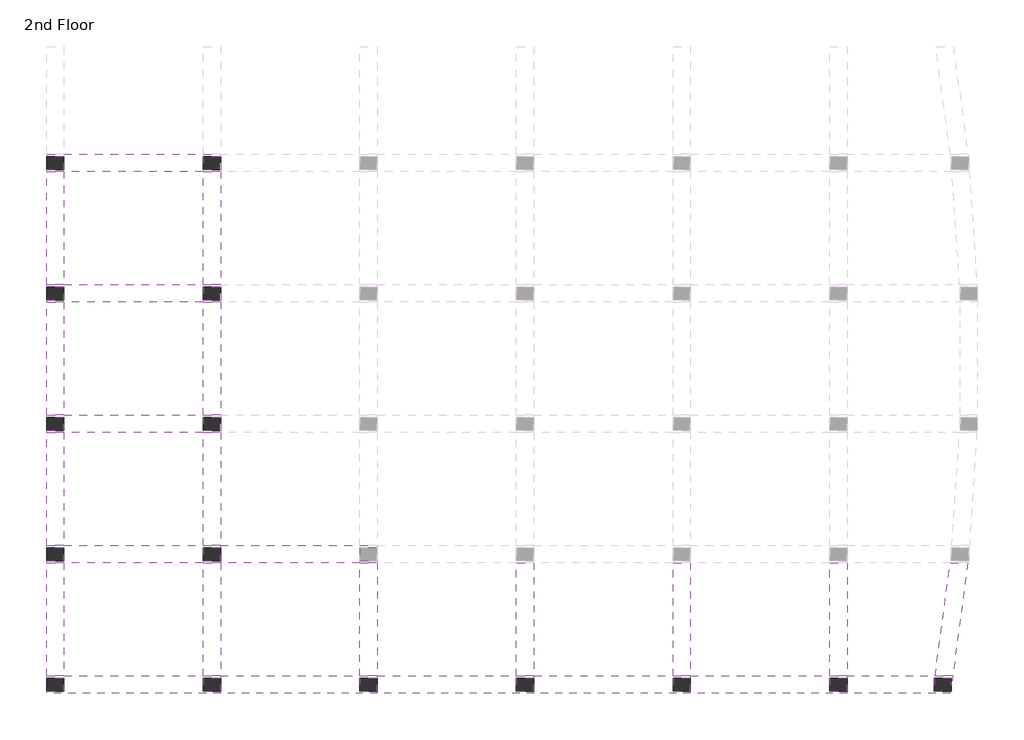
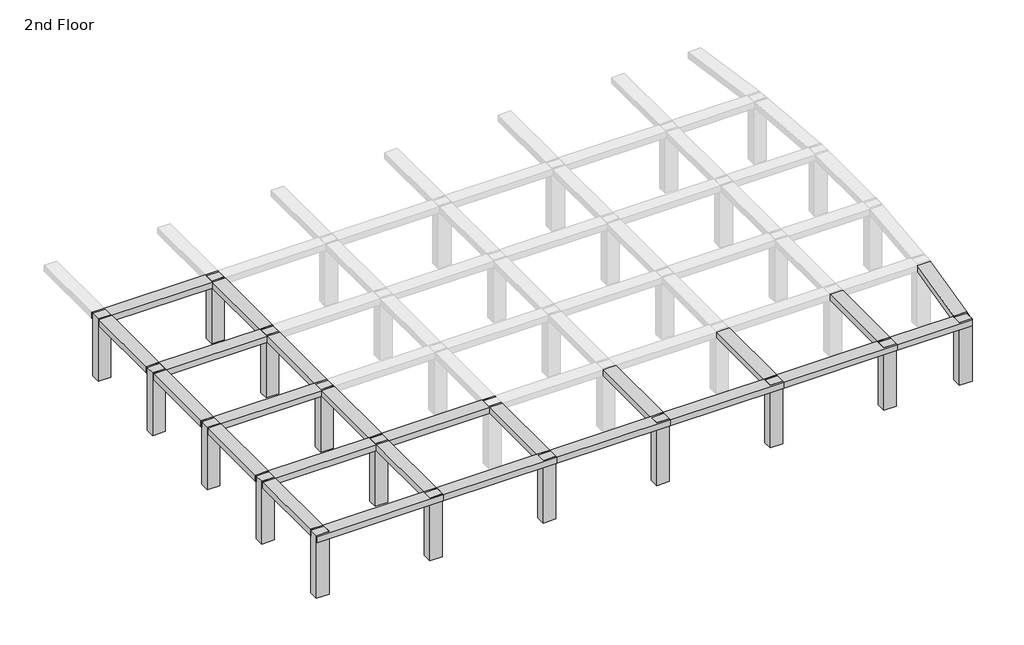
# One storey, part 1 of 3: 24 beams, 15 columns.
"""IFC4 building model written with IfcOpenShell, lengths in millimetres."""

from ifc_helpers import new_model, si_unit, frame, origin, place, context, project, spatial, polyline, outline, extrude, faceted_brep, element, save

model = new_model("IFC4")

# Units and contexts
model_context = context("Model", 3, world=origin())
ifc_project = project(units=[si_unit("LENGTHUNIT", "METRE", prefix="MILLI")], contexts=[model_context])

# Site, building, storey
site = spatial("IfcSite", under=ifc_project)
building = spatial("IfcBuilding", under=site)
storey = spatial("IfcBuildingStorey", under=building, Name="2nd Floor", Elevation=6400.8)

# Beams
placement = place(None, origin())
element("IfcBeam", 1, ObjectType="Concrete-Rectangular Beam : 2' x2'", at=placement, inside=storey, context=model_context, shape_type="Brep", body=[
    faceted_brep([(-16619.274232, -2891.2168778, 9601.2), (-17228.874232, -2891.2168778, 9601.2), (-22105.674232, -2891.2168778, 9601.2), (-22715.274232, -2891.2168778, 9601.2), (-22715.274232, -2967.4168778, 9601.2), (-22105.674232, -2967.4168778, 9601.2), (-22105.674232, -3424.6168778, 9601.2), (-22715.274232, -3424.6168778, 9601.2), (-22715.274232, -3500.8168778, 9601.2), (-16619.274232, -3500.8168778, 9601.2), (-16619.274232, -3424.6168778, 9601.2), (-17228.874232, -3424.6168778, 9601.2), (-17228.874232, -2967.4168778, 9601.2), (-16619.274232, -2967.4168778, 9601.2), (-22715.274232, -3500.8168778, 9296.4), (-16619.274232, -3500.8168778, 9296.4), (-22715.274232, -3424.6168778, 9296.4), (-22105.674232, -3424.6168778, 9296.4), (-22105.674232, -2967.4168778, 9296.4), (-22715.274232, -2967.4168778, 9296.4), (-22715.274232, -2891.2168778, 9296.4), (-22105.674232, -2891.2168778, 9296.4), (-17228.874232, -2891.2168778, 9296.4), (-16619.274232, -2891.2168778, 9296.4), (-16619.274232, -2967.4168778, 9296.4), (-17228.874232, -2967.4168778, 9296.4), (-17228.874232, -3424.6168778, 9296.4), (-16619.274232, -3424.6168778, 9296.4)], [[[0, 1, 2, 3, 4, 5, 6, 7, 8, 9, 10, 11, 12, 13]], [[8, 14, 15, 9]], [[15, 14, 16, 17, 18, 19, 20, 21, 22, 23, 24, 25, 26, 27]], [[20, 3, 2, 1, 0, 23, 22, 21]], [[14, 8, 7, 16]], [[9, 15, 27, 10]], [[17, 6, 5, 18]], [[6, 17, 16, 7]], [[18, 5, 4, 19]], [[3, 20, 19, 4]], [[26, 11, 10, 27]], [[11, 26, 25, 12]], [[12, 25, 24, 13]], [[23, 0, 13, 24]]]),
])
element("IfcBeam", 2, ObjectType="Concrete-Rectangular Beam : 2' x2'", at=placement, inside=storey, context=model_context, shape_type="Brep", body=[
    faceted_brep([(-16619.274232, -2891.2168778, 9601.2), (-16619.274232, -2967.4168778, 9601.2), (-16619.274232, -3424.6168778, 9601.2), (-16619.274232, -3500.8168778, 9601.2), (-11132.874232, -3500.8168778, 9601.2), (-11132.874232, -3424.6168778, 9601.2), (-11742.474232, -3424.6168778, 9601.2), (-11742.474232, -2967.4168778, 9601.2), (-11132.874232, -2967.4168778, 9601.2), (-11132.874232, -2891.2168778, 9601.2), (-11742.474232, -2891.2168778, 9601.2), (-11132.874232, -3500.8168778, 9296.4), (-16619.274232, -3500.8168778, 9296.4), (-16619.274232, -3424.6168778, 9296.4), (-16619.274232, -2967.4168778, 9296.4), (-16619.274232, -2891.2168778, 9296.4), (-11742.474232, -2891.2168778, 9296.4), (-11132.874232, -2891.2168778, 9296.4), (-11132.874232, -2967.4168778, 9296.4), (-11742.474232, -2967.4168778, 9296.4), (-11742.474232, -3424.6168778, 9296.4), (-11132.874232, -3424.6168778, 9296.4)], [[[0, 1, 2, 3, 4, 5, 6, 7, 8, 9, 10]], [[11, 4, 3, 12]], [[12, 13, 14, 15, 16, 17, 18, 19, 20, 21, 11]], [[15, 0, 10, 9, 17, 16]], [[3, 2, 1, 0, 15, 14, 13, 12]], [[4, 11, 21, 5]], [[20, 6, 5, 21]], [[6, 20, 19, 7]], [[7, 19, 18, 8]], [[17, 9, 8, 18]]]),
])
element("IfcBeam", 3, ObjectType="Concrete-Rectangular Beam : 2' x2'", at=placement, inside=storey, context=model_context, shape_type="Brep", body=[
    faceted_brep([(-5646.474232, -2891.2168778, 9601.2), (-6256.074232, -2891.2168778, 9601.2), (-11132.874232, -2891.2168778, 9601.2), (-11132.874232, -2967.4168778, 9601.2), (-11132.874232, -3424.6168778, 9601.2), (-11132.874232, -3500.8168778, 9601.2), (-5646.474232, -3500.8168778, 9601.2), (-5646.474232, -3424.6168778, 9601.2), (-6256.074232, -3424.6168778, 9601.2), (-6256.074232, -2967.4168778, 9601.2), (-5646.474232, -2967.4168778, 9601.2), (-5646.474232, -3500.8168778, 9296.4), (-11132.874232, -3500.8168778, 9296.4), (-11132.874232, -3424.6168778, 9296.4), (-11132.874232, -2967.4168778, 9296.4), (-11132.874232, -2891.2168778, 9296.4), (-6256.074232, -2891.2168778, 9296.4), (-5646.474232, -2891.2168778, 9296.4), (-5646.474232, -2967.4168778, 9296.4), (-6256.074232, -2967.4168778, 9296.4), (-6256.074232, -3424.6168778, 9296.4), (-5646.474232, -3424.6168778, 9296.4)], [[[0, 1, 2, 3, 4, 5, 6, 7, 8, 9, 10]], [[11, 6, 5, 12]], [[11, 12, 13, 14, 15, 16, 17, 18, 19, 20, 21]], [[0, 17, 16, 15, 2, 1]], [[6, 11, 21, 7]], [[5, 4, 3, 2, 15, 14, 13, 12]], [[20, 8, 7, 21]], [[8, 20, 19, 9]], [[9, 19, 18, 10]], [[17, 0, 10, 18]]]),
])
element("IfcBeam", 4, ObjectType="Concrete-Rectangular Beam : 2' x2'", at=placement, inside=storey, context=model_context, shape_type="Brep", body=[
    faceted_brep([(-5646.474232, -2891.2168778, 9601.2), (-5646.474232, -2967.4168778, 9601.2), (-5646.474232, -3424.6168778, 9601.2), (-5646.474232, -3500.8168778, 9601.2), (-160.074232, -3500.8168778, 9601.2), (-160.074232, -3424.6168778, 9601.2), (-769.674232, -3424.6168778, 9601.2), (-769.674232, -2967.4168778, 9601.2), (-160.074232, -2967.4168778, 9601.2), (-160.074232, -2891.2168778, 9601.2), (-769.674232, -2891.2168778, 9601.2), (-160.074232, -3500.8168778, 9296.4), (-5646.474232, -3500.8168778, 9296.4), (-5646.474232, -3424.6168778, 9296.4), (-5646.474232, -2967.4168778, 9296.4), (-5646.474232, -2891.2168778, 9296.4), (-769.674232, -2891.2168778, 9296.4), (-160.074232, -2891.2168778, 9296.4), (-160.074232, -2967.4168778, 9296.4), (-769.674232, -2967.4168778, 9296.4), (-769.674232, -3424.6168778, 9296.4), (-160.074232, -3424.6168778, 9296.4)], [[[0, 1, 2, 3, 4, 5, 6, 7, 8, 9, 10]], [[11, 4, 3, 12]], [[12, 13, 14, 15, 16, 17, 18, 19, 20, 21, 11]], [[15, 0, 10, 9, 17, 16]], [[3, 2, 1, 0, 15, 14, 13, 12]], [[4, 11, 21, 5]], [[20, 6, 5, 21]], [[6, 20, 19, 7]], [[7, 19, 18, 8]], [[17, 9, 8, 18]]]),
])
element("IfcBeam", 5, ObjectType="Concrete-Rectangular Beam : 2' x2'", at=placement, inside=storey, context=model_context, shape_type="Brep", body=[
    faceted_brep([(-160.074232, -2891.2168778, 9601.2), (-160.074232, -2967.4168778, 9601.2), (-160.074232, -3424.6168778, 9601.2), (-160.074232, -3500.8168778, 9601.2), (5326.325768, -3500.8168778, 9601.2), (5326.325768, -3424.6168778, 9601.2), (4716.725768, -3424.6168778, 9601.2), (4716.725768, -2967.4168778, 9601.2), (5326.325768, -2967.4168778, 9601.2), (5326.325768, -2891.2168778, 9601.2), (4716.725768, -2891.2168778, 9601.2), (5326.325768, -3500.8168778, 9296.4), (-160.074232, -3500.8168778, 9296.4), (-160.074232, -3424.6168778, 9296.4), (-160.074232, -2967.4168778, 9296.4), (-160.074232, -2891.2168778, 9296.4), (4716.725768, -2891.2168778, 9296.4), (5326.325768, -2891.2168778, 9296.4), (5326.325768, -2967.4168778, 9296.4), (4716.725768, -2967.4168778, 9296.4), (4716.725768, -3424.6168778, 9296.4), (5326.325768, -3424.6168778, 9296.4)], [[[0, 1, 2, 3, 4, 5, 6, 7, 8, 9, 10]], [[11, 4, 3, 12]], [[12, 13, 14, 15, 16, 17, 18, 19, 20, 21, 11]], [[15, 0, 10, 9, 17, 16]], [[3, 2, 1, 0, 15, 14, 13, 12]], [[4, 11, 21, 5]], [[20, 6, 5, 21]], [[6, 20, 19, 7]], [[7, 19, 18, 8]], [[17, 9, 8, 18]]]),
])
element("IfcBeam", 6, ObjectType="Concrete-Rectangular Beam : 2' x2'", at=placement, inside=storey, context=model_context, shape_type="Brep", body=[
    faceted_brep([(9027.2344863, -2891.2168778, 9601.2), (8412.2463849, -2891.2168778, 9601.2), (5326.325768, -2891.2168778, 9601.2), (5326.325768, -2967.4168778, 9601.2), (5326.325768, -3424.6168778, 9601.2), (5326.325768, -3500.8168778, 9601.2), (8946.005151, -3500.8168778, 9601.2), (8956.158818, -3424.6168778, 9601.2), (8374.325768, -3424.6168778, 9601.2), (8374.325768, -2967.4168778, 9601.2), (8983.925768, -2967.4168778, 9601.2), (8983.925768, -3216.2348608, 9601.2), (8946.005151, -3500.8168778, 9296.4), (5326.325768, -3500.8168778, 9296.4), (5326.325768, -3424.6168778, 9296.4), (5326.325768, -2967.4168778, 9296.4), (5326.325768, -2891.2168778, 9296.4), (8412.2463849, -2891.2168778, 9296.4), (9027.2344863, -2891.2168778, 9296.4), (8983.925768, -3216.2348608, 9296.4), (8983.925768, -2967.4168778, 9296.4), (8374.325768, -2967.4168778, 9296.4), (8374.325768, -3424.6168778, 9296.4), (8956.158818, -3424.6168778, 9296.4)], [[[0, 1, 2, 3, 4, 5, 6, 7, 8, 9, 10, 11]], [[12, 6, 5, 13]], [[12, 13, 14, 15, 16, 17, 18, 19, 20, 21, 22, 23]], [[0, 18, 17, 16, 2, 1]], [[6, 12, 23, 7]], [[5, 4, 3, 2, 16, 15, 14, 13]], [[10, 20, 19, 11]], [[22, 8, 7, 23]], [[8, 22, 21, 9]], [[9, 21, 20, 10]], [[18, 0, 11, 19]]]),
])
element("IfcBeam", 7, ObjectType="Concrete-Rectangular Beam : 2' x2'", at=placement, inside=storey, context=model_context, shape_type="Brep", body=[
    faceted_brep([(-16619.274232, 1680.7831222, 9601.2), (-17228.874232, 1680.7831222, 9601.2), (-22105.674232, 1680.7831222, 9601.2), (-22715.274232, 1680.7831222, 9601.2), (-22715.274232, 1604.5831222, 9601.2), (-22105.674232, 1604.5831222, 9601.2), (-22105.674232, 1147.3831222, 9601.2), (-22715.274232, 1147.3831222, 9601.2), (-22715.274232, 1071.1831222, 9601.2), (-22105.674232, 1071.1831222, 9601.2), (-17228.874232, 1071.1831222, 9601.2), (-16619.274232, 1071.1831222, 9601.2), (-16619.274232, 1147.3831222, 9601.2), (-17228.874232, 1147.3831222, 9601.2), (-17228.874232, 1604.5831222, 9601.2), (-16619.274232, 1604.5831222, 9601.2), (-22715.274232, 1071.1831222, 9296.4), (-22105.674232, 1071.1831222, 9296.4), (-17228.874232, 1071.1831222, 9296.4), (-16619.274232, 1071.1831222, 9296.4), (-22715.274232, 1147.3831222, 9296.4), (-22105.674232, 1147.3831222, 9296.4), (-22105.674232, 1604.5831222, 9296.4), (-22715.274232, 1604.5831222, 9296.4), (-22715.274232, 1680.7831222, 9296.4), (-22105.674232, 1680.7831222, 9296.4), (-17228.874232, 1680.7831222, 9296.4), (-16619.274232, 1680.7831222, 9296.4), (-16619.274232, 1604.5831222, 9296.4), (-17228.874232, 1604.5831222, 9296.4), (-17228.874232, 1147.3831222, 9296.4), (-16619.274232, 1147.3831222, 9296.4)], [[[0, 1, 2, 3, 4, 5, 6, 7, 8, 9, 10, 11, 12, 13, 14, 15]], [[8, 16, 17, 18, 19, 11, 10, 9]], [[19, 18, 17, 16, 20, 21, 22, 23, 24, 25, 26, 27, 28, 29, 30, 31]], [[24, 3, 2, 1, 0, 27, 26, 25]], [[16, 8, 7, 20]], [[11, 19, 31, 12]], [[21, 6, 5, 22]], [[6, 21, 20, 7]], [[22, 5, 4, 23]], [[3, 24, 23, 4]], [[30, 13, 12, 31]], [[13, 30, 29, 14]], [[14, 29, 28, 15]], [[27, 0, 15, 28]]]),
])
element("IfcBeam", 8, ObjectType="Concrete-Rectangular Beam : 2' x2'", at=placement, inside=storey, context=model_context, shape_type="Brep", body=[
    faceted_brep([(-16619.274232, 1680.7831222, 9601.2), (-16619.274232, 1604.5831222, 9601.2), (-16619.274232, 1147.3831222, 9601.2), (-16619.274232, 1071.1831222, 9601.2), (-11742.474232, 1071.1831222, 9601.2), (-11132.874232, 1071.1831222, 9601.2), (-11132.874232, 1147.3831222, 9601.2), (-11742.474232, 1147.3831222, 9601.2), (-11742.474232, 1604.5831222, 9601.2), (-11132.874232, 1604.5831222, 9601.2), (-11132.874232, 1680.7831222, 9601.2), (-11742.474232, 1680.7831222, 9601.2), (-16619.274232, 1071.1831222, 9296.4), (-11742.474232, 1071.1831222, 9296.4), (-11132.874232, 1071.1831222, 9296.4), (-16619.274232, 1147.3831222, 9296.4), (-16619.274232, 1604.5831222, 9296.4), (-16619.274232, 1680.7831222, 9296.4), (-11742.474232, 1680.7831222, 9296.4), (-11132.874232, 1680.7831222, 9296.4), (-11132.874232, 1604.5831222, 9296.4), (-11742.474232, 1604.5831222, 9296.4), (-11742.474232, 1147.3831222, 9296.4), (-11132.874232, 1147.3831222, 9296.4)], [[[0, 1, 2, 3, 4, 5, 6, 7, 8, 9, 10, 11]], [[3, 12, 13, 14, 5, 4]], [[12, 15, 16, 17, 18, 19, 20, 21, 22, 23, 14, 13]], [[10, 19, 18, 17, 0, 11]], [[3, 2, 1, 0, 17, 16, 15, 12]], [[5, 14, 23, 6]], [[22, 7, 6, 23]], [[7, 22, 21, 8]], [[8, 21, 20, 9]], [[19, 10, 9, 20]]]),
])
element("IfcBeam", 9, ObjectType="Concrete-Rectangular Beam : 2' x2'", at=placement, inside=storey, context=model_context, shape_type="Brep", body=[
    faceted_brep([(-16619.274232, 6252.7831222, 9601.2), (-17228.874232, 6252.7831222, 9601.2), (-22105.674232, 6252.7831222, 9601.2), (-22715.274232, 6252.7831222, 9601.2), (-22715.274232, 6176.5831222, 9601.2), (-22105.674232, 6176.5831222, 9601.2), (-22105.674232, 5719.3831222, 9601.2), (-22715.274232, 5719.3831222, 9601.2), (-22715.274232, 5643.1831222, 9601.2), (-22105.674232, 5643.1831222, 9601.2), (-17228.874232, 5643.1831222, 9601.2), (-16619.274232, 5643.1831222, 9601.2), (-16619.274232, 5719.3831222, 9601.2), (-17228.874232, 5719.3831222, 9601.2), (-17228.874232, 6176.5831222, 9601.2), (-16619.274232, 6176.5831222, 9601.2), (-22715.274232, 5643.1831222, 9296.4), (-22105.674232, 5643.1831222, 9296.4), (-17228.874232, 5643.1831222, 9296.4), (-16619.274232, 5643.1831222, 9296.4), (-22715.274232, 5719.3831222, 9296.4), (-22105.674232, 5719.3831222, 9296.4), (-22105.674232, 6176.5831222, 9296.4), (-22715.274232, 6176.5831222, 9296.4), (-22715.274232, 6252.7831222, 9296.4), (-22105.674232, 6252.7831222, 9296.4), (-17228.874232, 6252.7831222, 9296.4), (-16619.274232, 6252.7831222, 9296.4), (-16619.274232, 6176.5831222, 9296.4), (-17228.874232, 6176.5831222, 9296.4), (-17228.874232, 5719.3831222, 9296.4), (-16619.274232, 5719.3831222, 9296.4)], [[[0, 1, 2, 3, 4, 5, 6, 7, 8, 9, 10, 11, 12, 13, 14, 15]], [[8, 16, 17, 18, 19, 11, 10, 9]], [[19, 18, 17, 16, 20, 21, 22, 23, 24, 25, 26, 27, 28, 29, 30, 31]], [[24, 3, 2, 1, 0, 27, 26, 25]], [[16, 8, 7, 20]], [[11, 19, 31, 12]], [[21, 6, 5, 22]], [[6, 21, 20, 7]], [[22, 5, 4, 23]], [[3, 24, 23, 4]], [[30, 13, 12, 31]], [[13, 30, 29, 14]], [[14, 29, 28, 15]], [[27, 0, 15, 28]]]),
])
element("IfcBeam", 10, ObjectType="Concrete-Rectangular Beam : 2' x2'", at=placement, inside=storey, context=model_context, shape_type="Brep", body=[
    faceted_brep([(-16619.274232, 10824.7831222, 9601.2), (-17228.874232, 10824.7831222, 9601.2), (-22105.674232, 10824.7831222, 9601.2), (-22715.274232, 10824.7831222, 9601.2), (-22715.274232, 10748.5831222, 9601.2), (-22105.674232, 10748.5831222, 9601.2), (-22105.674232, 10291.3831222, 9601.2), (-22715.274232, 10291.3831222, 9601.2), (-22715.274232, 10215.1831222, 9601.2), (-22105.674232, 10215.1831222, 9601.2), (-17228.874232, 10215.1831222, 9601.2), (-16619.274232, 10215.1831222, 9601.2), (-16619.274232, 10291.3831222, 9601.2), (-17228.874232, 10291.3831222, 9601.2), (-17228.874232, 10748.5831222, 9601.2), (-16619.274232, 10748.5831222, 9601.2), (-22715.274232, 10215.1831222, 9296.4), (-22105.674232, 10215.1831222, 9296.4), (-17228.874232, 10215.1831222, 9296.4), (-16619.274232, 10215.1831222, 9296.4), (-22715.274232, 10291.3831222, 9296.4), (-22105.674232, 10291.3831222, 9296.4), (-22105.674232, 10748.5831222, 9296.4), (-22715.274232, 10748.5831222, 9296.4), (-22715.274232, 10824.7831222, 9296.4), (-22105.674232, 10824.7831222, 9296.4), (-17228.874232, 10824.7831222, 9296.4), (-16619.274232, 10824.7831222, 9296.4), (-16619.274232, 10748.5831222, 9296.4), (-17228.874232, 10748.5831222, 9296.4), (-17228.874232, 10291.3831222, 9296.4), (-16619.274232, 10291.3831222, 9296.4)], [[[0, 1, 2, 3, 4, 5, 6, 7, 8, 9, 10, 11, 12, 13, 14, 15]], [[8, 16, 17, 18, 19, 11, 10, 9]], [[19, 18, 17, 16, 20, 21, 22, 23, 24, 25, 26, 27, 28, 29, 30, 31]], [[24, 3, 2, 1, 0, 27, 26, 25]], [[16, 8, 7, 20]], [[11, 19, 31, 12]], [[21, 6, 5, 22]], [[6, 21, 20, 7]], [[22, 5, 4, 23]], [[3, 24, 23, 4]], [[30, 13, 12, 31]], [[13, 30, 29, 14]], [[14, 29, 28, 15]], [[27, 0, 15, 28]]]),
])
element("IfcBeam", 11, ObjectType="Concrete-Rectangular Beam : 2' x2'", at=placement, inside=storey, context=model_context, shape_type="Brep", body=[
    faceted_brep([(-16619.274232, 15396.7831222, 9601.2), (-17228.874232, 15396.7831222, 9601.2), (-22105.674232, 15396.7831222, 9601.2), (-22715.274232, 15396.7831222, 9601.2), (-22715.274232, 15320.5831222, 9601.2), (-22105.674232, 15320.5831222, 9601.2), (-22105.674232, 14863.3831222, 9601.2), (-22715.274232, 14863.3831222, 9601.2), (-22715.274232, 14787.1831222, 9601.2), (-22105.674232, 14787.1831222, 9601.2), (-17228.874232, 14787.1831222, 9601.2), (-16619.274232, 14787.1831222, 9601.2), (-16619.274232, 14863.3831222, 9601.2), (-17228.874232, 14863.3831222, 9601.2), (-17228.874232, 15320.5831222, 9601.2), (-16619.274232, 15320.5831222, 9601.2), (-22715.274232, 14787.1831222, 9296.4), (-22105.674232, 14787.1831222, 9296.4), (-17228.874232, 14787.1831222, 9296.4), (-16619.274232, 14787.1831222, 9296.4), (-22715.274232, 14863.3831222, 9296.4), (-22105.674232, 14863.3831222, 9296.4), (-22105.674232, 15320.5831222, 9296.4), (-22715.274232, 15320.5831222, 9296.4), (-22715.274232, 15396.7831222, 9296.4), (-22105.674232, 15396.7831222, 9296.4), (-17228.874232, 15396.7831222, 9296.4), (-16619.274232, 15396.7831222, 9296.4), (-16619.274232, 15320.5831222, 9296.4), (-17228.874232, 15320.5831222, 9296.4), (-17228.874232, 14863.3831222, 9296.4), (-16619.274232, 14863.3831222, 9296.4)], [[[0, 1, 2, 3, 4, 5, 6, 7, 8, 9, 10, 11, 12, 13, 14, 15]], [[8, 16, 17, 18, 19, 11, 10, 9]], [[19, 18, 17, 16, 20, 21, 22, 23, 24, 25, 26, 27, 28, 29, 30, 31]], [[24, 3, 2, 1, 0, 27, 26, 25]], [[16, 8, 7, 20]], [[11, 19, 31, 12]], [[21, 6, 5, 22]], [[6, 21, 20, 7]], [[22, 5, 4, 23]], [[3, 24, 23, 4]], [[30, 13, 12, 31]], [[13, 30, 29, 14]], [[14, 29, 28, 15]], [[27, 0, 15, 28]]]),
])
element("IfcBeam", 12, ObjectType="Concrete-Rectangular Beam : 2' x2'", at=placement, inside=storey, context=model_context, shape_type="SweptSolid", body=[
    extrude(outline(polyline([(-22105.674232, -2891.2168778), (-22715.274232, -2891.2168778), (-22715.274232, 1071.1831222), (-22105.674232, 1071.1831222), (-22105.674232, -2891.2168778)])), frame((0.0, 0.0, 9296.4), z_axis=(0.0, 0.0, 1.0), x_axis=(1.0, 0.0, 0.0)), (0.0, 0.0, 1.0), 304.8),
])
element("IfcBeam", 13, ObjectType="Concrete-Rectangular Beam : 2' x2'", at=placement, inside=storey, context=model_context, shape_type="SweptSolid", body=[
    extrude(outline(polyline([(-22105.674232, 1680.7831222), (-22715.274232, 1680.7831222), (-22715.274232, 5643.1831222), (-22105.674232, 5643.1831222), (-22105.674232, 1680.7831222)])), frame((0.0, 0.0, 9296.4), z_axis=(0.0, 0.0, 1.0), x_axis=(1.0, 0.0, 0.0)), (0.0, 0.0, 1.0), 304.8),
])
element("IfcBeam", 14, ObjectType="Concrete-Rectangular Beam : 2' x2'", at=placement, inside=storey, context=model_context, shape_type="SweptSolid", body=[
    extrude(outline(polyline([(-22105.674232, 6252.7831222), (-22715.274232, 6252.7831222), (-22715.274232, 10215.1831222), (-22105.674232, 10215.1831222), (-22105.674232, 6252.7831222)])), frame((0.0, 0.0, 9296.4), z_axis=(0.0, 0.0, 1.0), x_axis=(1.0, 0.0, 0.0)), (0.0, 0.0, 1.0), 304.8),
])
element("IfcBeam", 15, ObjectType="Concrete-Rectangular Beam : 2' x2'", at=placement, inside=storey, context=model_context, shape_type="SweptSolid", body=[
    extrude(outline(polyline([(-22105.674232, 10824.7831222), (-22715.274232, 10824.7831222), (-22715.274232, 14787.1831222), (-22105.674232, 14787.1831222), (-22105.674232, 10824.7831222)])), frame((0.0, 0.0, 9296.4), z_axis=(0.0, 0.0, 1.0), x_axis=(1.0, 0.0, 0.0)), (0.0, 0.0, 1.0), 304.8),
])
element("IfcBeam", 16, ObjectType="Concrete-Rectangular Beam : 2' x2'", at=placement, inside=storey, context=model_context, shape_type="SweptSolid", body=[
    extrude(outline(polyline([(-17228.874232, 1071.1831222), (-16619.274232, 1071.1831222), (-16619.274232, -2891.2168778), (-17228.874232, -2891.2168778), (-17228.874232, 1071.1831222)])), frame((0.0, 0.0, 9296.4), z_axis=(0.0, 0.0, 1.0), x_axis=(1.0, 0.0, 0.0)), (0.0, 0.0, 1.0), 304.8),
])
element("IfcBeam", 17, ObjectType="Concrete-Rectangular Beam : 2' x2'", at=placement, inside=storey, context=model_context, shape_type="SweptSolid", body=[
    extrude(outline(polyline([(-16619.274232, 1680.7831222), (-17228.874232, 1680.7831222), (-17228.874232, 5643.1831222), (-16619.274232, 5643.1831222), (-16619.274232, 1680.7831222)])), frame((0.0, 0.0, 9296.4), z_axis=(0.0, 0.0, 1.0), x_axis=(1.0, 0.0, 0.0)), (0.0, 0.0, 1.0), 304.8),
])
element("IfcBeam", 18, ObjectType="Concrete-Rectangular Beam : 2' x2'", at=placement, inside=storey, context=model_context, shape_type="SweptSolid", body=[
    extrude(outline(polyline([(-16619.274232, 6252.7831222), (-17228.874232, 6252.7831222), (-17228.874232, 10215.1831222), (-16619.274232, 10215.1831222), (-16619.274232, 6252.7831222)])), frame((0.0, 0.0, 9296.4), z_axis=(0.0, 0.0, 1.0), x_axis=(1.0, 0.0, 0.0)), (0.0, 0.0, 1.0), 304.8),
])
element("IfcBeam", 19, ObjectType="Concrete-Rectangular Beam : 2' x2'", at=placement, inside=storey, context=model_context, shape_type="SweptSolid", body=[
    extrude(outline(polyline([(-16619.274232, 10824.7831222), (-17228.874232, 10824.7831222), (-17228.874232, 14787.1831222), (-16619.274232, 14787.1831222), (-16619.274232, 10824.7831222)])), frame((0.0, 0.0, 9296.4), z_axis=(0.0, 0.0, 1.0), x_axis=(1.0, 0.0, 0.0)), (0.0, 0.0, 1.0), 304.8),
])
element("IfcBeam", 20, ObjectType="Concrete-Rectangular Beam : 2' x2'", at=placement, inside=storey, context=model_context, shape_type="SweptSolid", body=[
    extrude(outline(polyline([(-11742.474232, 1071.1831222), (-11132.874232, 1071.1831222), (-11132.874232, -2891.2168778), (-11742.474232, -2891.2168778), (-11742.474232, 1071.1831222)])), frame((0.0, 0.0, 9296.4), z_axis=(0.0, 0.0, 1.0), x_axis=(1.0, 0.0, 0.0)), (0.0, 0.0, 1.0), 304.8),
])
element("IfcBeam", 21, ObjectType="Concrete-Rectangular Beam : 2' x2'", at=placement, inside=storey, context=model_context, shape_type="SweptSolid", body=[
    extrude(outline(polyline([(-6256.074232, 1071.1831222), (-5646.474232, 1071.1831222), (-5646.474232, -2891.2168778), (-6256.074232, -2891.2168778), (-6256.074232, 1071.1831222)])), frame((0.0, 0.0, 9296.4), z_axis=(0.0, 0.0, 1.0), x_axis=(1.0, 0.0, 0.0)), (0.0, 0.0, 1.0), 304.8),
])
element("IfcBeam", 22, ObjectType="Concrete-Rectangular Beam : 2' x2'", at=placement, inside=storey, context=model_context, shape_type="SweptSolid", body=[
    extrude(outline(polyline([(-769.674232, 1071.1831222), (-160.074232, 1071.1831222), (-160.074232, -2891.2168778), (-769.674232, -2891.2168778), (-769.674232, 1071.1831222)])), frame((0.0, 0.0, 9296.4), z_axis=(0.0, 0.0, 1.0), x_axis=(1.0, 0.0, 0.0)), (0.0, 0.0, 1.0), 304.8),
])
element("IfcBeam", 23, ObjectType="Concrete-Rectangular Beam : 2' x2'", at=placement, inside=storey, context=model_context, shape_type="SweptSolid", body=[
    extrude(outline(polyline([(4716.725768, 1071.1831222), (5326.325768, 1071.1831222), (5326.325768, -2891.2168778), (4716.725768, -2891.2168778), (4716.725768, 1071.1831222)])), frame((0.0, 0.0, 9296.4), z_axis=(0.0, 0.0, 1.0), x_axis=(1.0, 0.0, 0.0)), (0.0, 0.0, 1.0), 304.8),
])
element("IfcBeam", 24, ObjectType="Concrete-Rectangular Beam : 2' x2'", at=placement, inside=storey, context=model_context, shape_type="SweptSolid", body=[
    extrude(outline(polyline([(8940.2370643, 1071.1831222), (9555.2251658, 1071.1831222), (9027.2344863, -2891.2168778), (8412.2463849, -2891.2168778), (8940.2370643, 1071.1831222)])), frame((0.0, 0.0, 9296.4), z_axis=(0.0, 0.0, 1.0), x_axis=(1.0, 0.0, 0.0)), (0.0, 0.0, 1.0), 304.8),
])

# Columns
element("IfcColumn", 25, ObjectType="Concrete-Rectangular-Column : 12 x 18", at=placement, inside=storey, context=model_context, shape_type="SweptSolid", body=[
    extrude(outline(polyline([(-22105.674232, -2967.4168778), (-22105.674232, -3424.6168778), (-22715.274232, -3424.6168778), (-22715.274232, -2967.4168778), (-22105.674232, -2967.4168778)])), frame((0.0, 0.0, 6400.8), z_axis=(0.0, 0.0, 1.0), x_axis=(1.0, 0.0, 0.0)), (0.0, 0.0, 1.0), 3200.4),
])
element("IfcColumn", 26, ObjectType="Concrete-Rectangular-Column : 12 x 18", at=placement, inside=storey, context=model_context, shape_type="SweptSolid", body=[
    extrude(outline(polyline([(-16619.274232, -2967.4168778), (-16619.274232, -3424.6168778), (-17228.874232, -3424.6168778), (-17228.874232, -2967.4168778), (-16619.274232, -2967.4168778)])), frame((0.0, 0.0, 6400.8), z_axis=(0.0, 0.0, 1.0), x_axis=(1.0, 0.0, 0.0)), (0.0, 0.0, 1.0), 3200.4),
])
element("IfcColumn", 27, ObjectType="Concrete-Rectangular-Column : 12 x 18", at=placement, inside=storey, context=model_context, shape_type="SweptSolid", body=[
    extrude(outline(polyline([(-11132.874232, -2967.4168778), (-11132.874232, -3424.6168778), (-11742.474232, -3424.6168778), (-11742.474232, -2967.4168778), (-11132.874232, -2967.4168778)])), frame((0.0, 0.0, 6400.8), z_axis=(0.0, 0.0, 1.0), x_axis=(1.0, 0.0, 0.0)), (0.0, 0.0, 1.0), 3200.4),
])
element("IfcColumn", 28, ObjectType="Concrete-Rectangular-Column : 12 x 18", at=placement, inside=storey, context=model_context, shape_type="SweptSolid", body=[
    extrude(outline(polyline([(-5646.474232, -2967.4168778), (-5646.474232, -3424.6168778), (-6256.074232, -3424.6168778), (-6256.074232, -2967.4168778), (-5646.474232, -2967.4168778)])), frame((0.0, 0.0, 6400.8), z_axis=(0.0, 0.0, 1.0), x_axis=(1.0, 0.0, 0.0)), (0.0, 0.0, 1.0), 3200.4),
])
element("IfcColumn", 29, ObjectType="Concrete-Rectangular-Column : 12 x 18", at=placement, inside=storey, context=model_context, shape_type="SweptSolid", body=[
    extrude(outline(polyline([(-160.074232, -2967.4168778), (-160.074232, -3424.6168778), (-769.674232, -3424.6168778), (-769.674232, -2967.4168778), (-160.074232, -2967.4168778)])), frame((0.0, 0.0, 6400.8), z_axis=(0.0, 0.0, 1.0), x_axis=(1.0, 0.0, 0.0)), (0.0, 0.0, 1.0), 3200.4),
])
element("IfcColumn", 30, ObjectType="Concrete-Rectangular-Column : 12 x 18", at=placement, inside=storey, context=model_context, shape_type="SweptSolid", body=[
    extrude(outline(polyline([(5326.325768, -2967.4168778), (5326.325768, -3424.6168778), (4716.725768, -3424.6168778), (4716.725768, -2967.4168778), (5326.325768, -2967.4168778)])), frame((0.0, 0.0, 6400.8), z_axis=(0.0, 0.0, 1.0), x_axis=(1.0, 0.0, 0.0)), (0.0, 0.0, 1.0), 3200.4),
])
element("IfcColumn", 31, ObjectType="Concrete-Rectangular-Column : 12 x 18", at=placement, inside=storey, context=model_context, shape_type="SweptSolid", body=[
    extrude(outline(polyline([(8983.925768, -2967.4168778), (8983.925768, -3424.6168778), (8374.325768, -3424.6168778), (8374.325768, -2967.4168778), (8983.925768, -2967.4168778)])), frame((0.0, 0.0, 6400.8), z_axis=(0.0, 0.0, 1.0), x_axis=(1.0, 0.0, 0.0)), (0.0, 0.0, 1.0), 3200.4),
])
element("IfcColumn", 32, ObjectType="Concrete-Rectangular-Column : 12 x 18", at=placement, inside=storey, context=model_context, shape_type="SweptSolid", body=[
    extrude(outline(polyline([(-22105.674232, 1604.5831222), (-22105.674232, 1147.3831222), (-22715.274232, 1147.3831222), (-22715.274232, 1604.5831222), (-22105.674232, 1604.5831222)])), frame((0.0, 0.0, 6400.8), z_axis=(0.0, 0.0, 1.0), x_axis=(1.0, 0.0, 0.0)), (0.0, 0.0, 1.0), 3200.4),
])
element("IfcColumn", 33, ObjectType="Concrete-Rectangular-Column : 12 x 18", at=placement, inside=storey, context=model_context, shape_type="SweptSolid", body=[
    extrude(outline(polyline([(-16619.274232, 1604.5831222), (-16619.274232, 1147.3831222), (-17228.874232, 1147.3831222), (-17228.874232, 1604.5831222), (-16619.274232, 1604.5831222)])), frame((0.0, 0.0, 6400.8), z_axis=(0.0, 0.0, 1.0), x_axis=(1.0, 0.0, 0.0)), (0.0, 0.0, 1.0), 3200.4),
])
element("IfcColumn", 34, ObjectType="Concrete-Rectangular-Column : 12 x 18", at=placement, inside=storey, context=model_context, shape_type="SweptSolid", body=[
    extrude(outline(polyline([(-22105.674232, 6176.5831222), (-22105.674232, 5719.3831222), (-22715.274232, 5719.3831222), (-22715.274232, 6176.5831222), (-22105.674232, 6176.5831222)])), frame((0.0, 0.0, 6400.8), z_axis=(0.0, 0.0, 1.0), x_axis=(1.0, 0.0, 0.0)), (0.0, 0.0, 1.0), 3200.4),
])
element("IfcColumn", 35, ObjectType="Concrete-Rectangular-Column : 12 x 18", at=placement, inside=storey, context=model_context, shape_type="SweptSolid", body=[
    extrude(outline(polyline([(-16619.274232, 6176.5831222), (-16619.274232, 5719.3831222), (-17228.874232, 5719.3831222), (-17228.874232, 6176.5831222), (-16619.274232, 6176.5831222)])), frame((0.0, 0.0, 6400.8), z_axis=(0.0, 0.0, 1.0), x_axis=(1.0, 0.0, 0.0)), (0.0, 0.0, 1.0), 3200.4),
])
element("IfcColumn", 36, ObjectType="Concrete-Rectangular-Column : 12 x 18", at=placement, inside=storey, context=model_context, shape_type="SweptSolid", body=[
    extrude(outline(polyline([(-22105.674232, 10748.5831222), (-22105.674232, 10291.3831222), (-22715.274232, 10291.3831222), (-22715.274232, 10748.5831222), (-22105.674232, 10748.5831222)])), frame((0.0, 0.0, 6400.8), z_axis=(0.0, 0.0, 1.0), x_axis=(1.0, 0.0, 0.0)), (0.0, 0.0, 1.0), 3200.4),
])
element("IfcColumn", 37, ObjectType="Concrete-Rectangular-Column : 12 x 18", at=placement, inside=storey, context=model_context, shape_type="SweptSolid", body=[
    extrude(outline(polyline([(-16619.274232, 10748.5831222), (-16619.274232, 10291.3831222), (-17228.874232, 10291.3831222), (-17228.874232, 10748.5831222), (-16619.274232, 10748.5831222)])), frame((0.0, 0.0, 6400.8), z_axis=(0.0, 0.0, 1.0), x_axis=(1.0, 0.0, 0.0)), (0.0, 0.0, 1.0), 3200.4),
])
element("IfcColumn", 38, ObjectType="Concrete-Rectangular-Column : 12 x 18", at=placement, inside=storey, context=model_context, shape_type="SweptSolid", body=[
    extrude(outline(polyline([(-22105.674232, 15320.5831222), (-22105.674232, 14863.3831222), (-22715.274232, 14863.3831222), (-22715.274232, 15320.5831222), (-22105.674232, 15320.5831222)])), frame((0.0, 0.0, 6400.8), z_axis=(0.0, 0.0, 1.0), x_axis=(1.0, 0.0, 0.0)), (0.0, 0.0, 1.0), 3200.4),
])
element("IfcColumn", 39, ObjectType="Concrete-Rectangular-Column : 12 x 18", at=placement, inside=storey, context=model_context, shape_type="SweptSolid", body=[
    extrude(outline(polyline([(-16619.274232, 15320.5831222), (-16619.274232, 14863.3831222), (-17228.874232, 14863.3831222), (-17228.874232, 15320.5831222), (-16619.274232, 15320.5831222)])), frame((0.0, 0.0, 6400.8), z_axis=(0.0, 0.0, 1.0), x_axis=(1.0, 0.0, 0.0)), (0.0, 0.0, 1.0), 3200.4),
])

save(model, "model.ifc")

# Revit data of these elements
# Type "Concrete-Rectangular Beam : 2' x2'"
#   Assembly Code = "B10"
#   Length [instance default] = 5' - 0"
#   b = 2' - 0"
#   h = 1' - 0"
#   Structural Material [instance default] = Concrete, Cast-in-Place gray
# Type "Concrete-Rectangular-Column : 12 x 18"
#   Assembly Code = "B10"
#   b = 2' - 0"
#   h = 1' - 6"
#   Structural Material [instance default] = Concrete, Cast-in-Place gray
# Elements 1, 2, 3, 4, 5, 6, 7, 8, 9, 10, 11, 12, 13, 14, 15, 16, 17, 18, 19, 20, 21, 22, 23, 24 (IfcBeam, "Concrete-Rectangular Beam : 2' x2'")
#   Structural Material = Concrete, Precast (2)
#   Phase Created = New Construction
#   Materials on its faces: "Concrete, Precast (2)"
# Elements 25, 26, 27, 28, 29, 30, 31, 32, 33, 34, 35, 36, 37, 38, 39 (IfcColumn, "Concrete-Rectangular-Column : 12 x 18")
#   Phase Created = New Construction
#   Materials on its faces: "Concrete, Cast-in-Place gray"
# Materials
#   "Concrete, Cast-in-Place gray": class "Concrete", colour RGB 192 192 192, transparency 0, Description = "Cast-in-place concrete", Cost = 0
#   "Concrete, Precast (2)": class "Concrete", colour RGB 198 187 187, transparency 0, Description = "Precast concrete", Cost = 0
